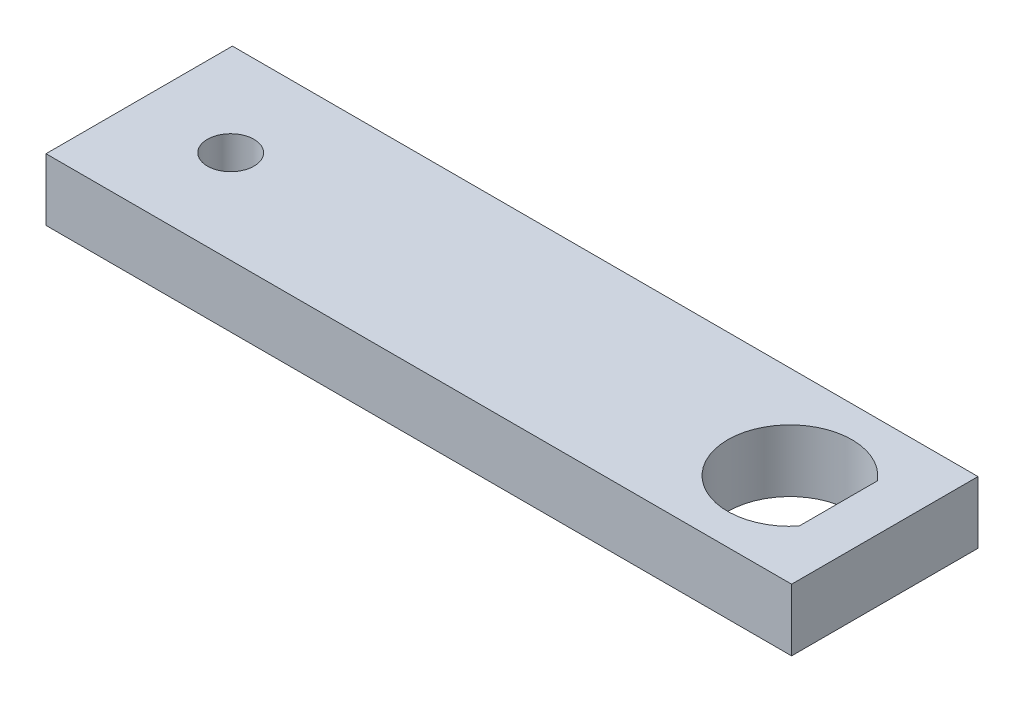
SolidWorks part; units mm, degrees
material "Plain Carbon Steel"
ref_plane "Front Plane" through (0, 0, 0) normal (0, 0, 1) x (1, 0, 0)
ref_plane "Top Plane" through (0, 0, 0) normal (0, 1, 0) x (1, 0, 0)
ref_plane "Right Plane" through (0, 0, 0) normal (1, 0, 0) x (0, 0, -1)
sketch "Bar Outline and Hole Ø4.76 Sketch" plane through (0, 0, 0) normal (0, 1, 0) x (1, 0, 0)
  line L1 (-38.1, 9.525) -> (38.1, 9.525)
  line L2 (-38.1, 9.525) -> (-38.1, -9.525)
  line L3 (-38.1, -9.525) -> (38.1, -9.525)
  line L4 (38.1, 9.525) -> (38.1, -9.525)
  line L5 (-38.1, 9.525) -> (38.1, -9.525) construction
  line L6 (-38.1, -9.525) -> (38.1, 9.525) construction
  circle A0 centre (-28.75, 0) radius 2.38
  point P0 (0, 0)
  dimension "D4" = 4.76
  dimension "D1" = 19.05
  dimension "D2" = 76.2
  dimension "D3" = 9.35
extrude "Link Bar 6.35 Thick" add sketch "Bar Outline and Hole Ø4.76 Sketch" along normal blind 6.35
sketch "D-Hole Ø12.7 Sketch" plane through (0, 6.35, 0) normal (0, 1, 0) x (1, 0, 0)
  line L0 (38.1, -9.525) -> (38.1, 9.525) construction
  line L1 (33.34, -3.9898) -> (33.34, 3.9898)
  arc A0 (33.34, 3.9898) -> (33.34, -3.9898) centre (28.4, 0) ccw
  dimension "D1" = 12.7
  dimension "D2" = 9.7
  dimension "D3" = 4.76
extrude "D-Hole Ø12.7 Cut" cut sketch "D-Hole Ø12.7 Sketch" against normal blind 6.35
